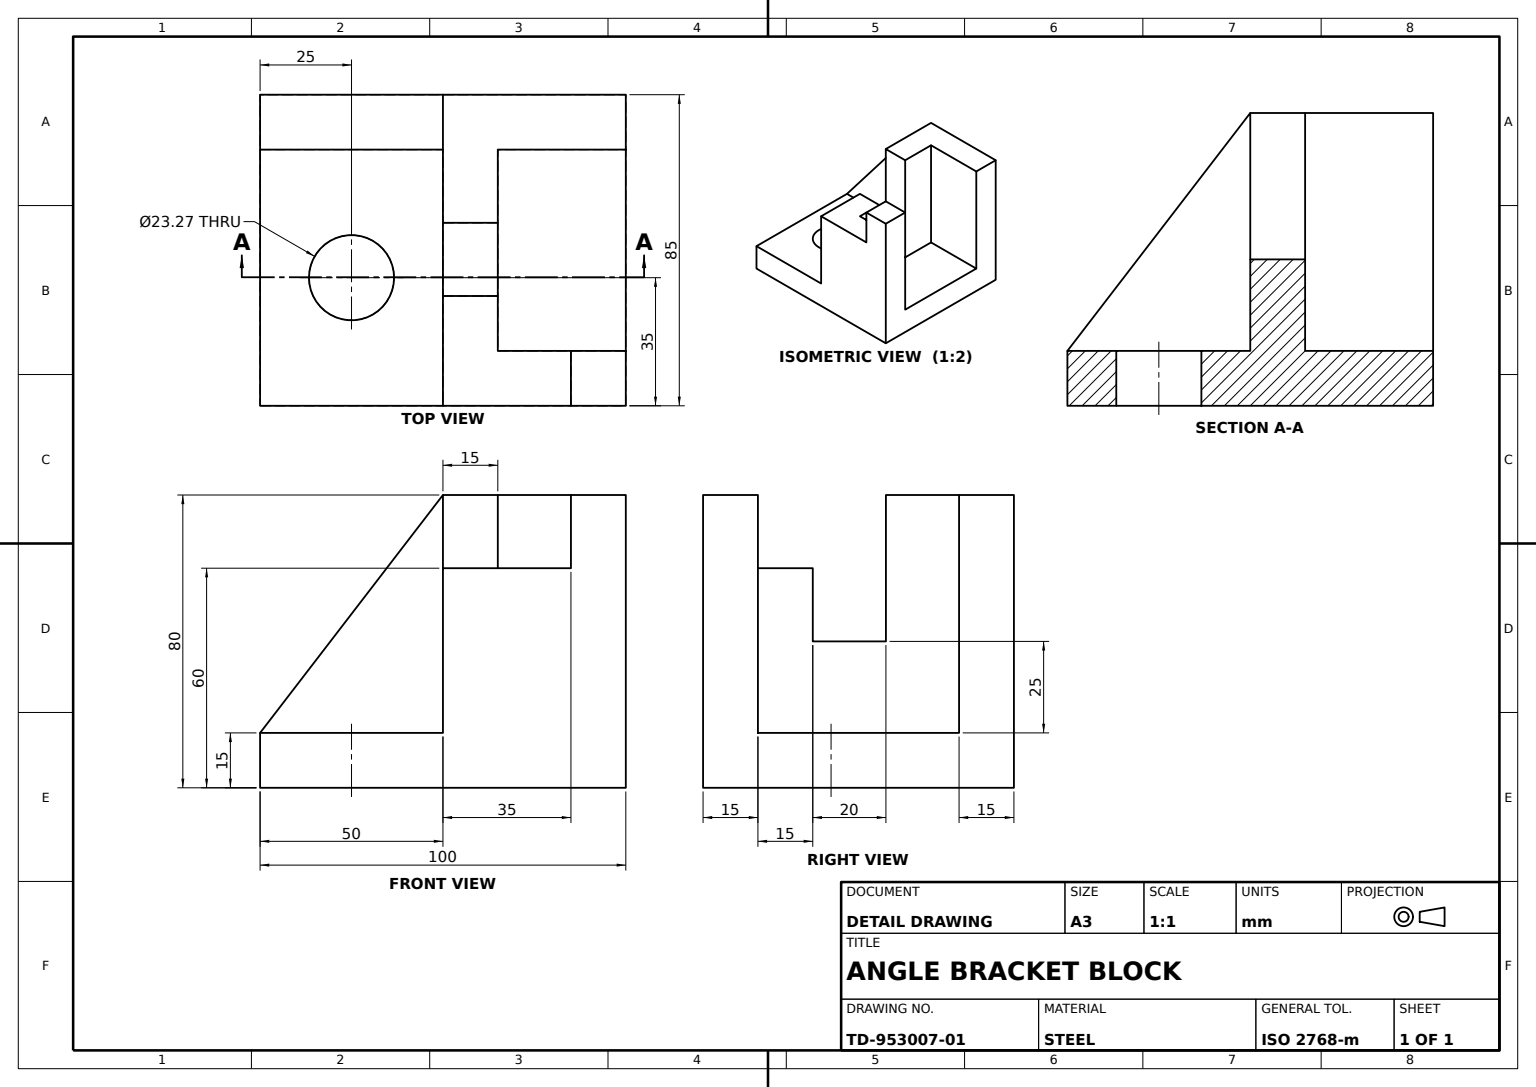
from build123d import *

# Parameters (mm, degrees)
BASE_PLATE_SKETCH_W    = 85
BASE_PLATE_SKETCH_H    = 100
BASE_PLATE_DEPTH       = 15
UPRIGHT_WALL_DEPTH     = 15
SIDE_WALL_SKETCH_W     = 50
SIDE_WALL_SKETCH_H     = 65
SIDE_WALL_DEPTH        = 15
GUSSET_DEPTH           = 15
POST_SKETCH_W          = 20
POST_SKETCH_H          = 15
POST_DEPTH             = 60
STEPPED_BLOCK_DEPTH    = 15
MOUNTING_HOLE_SKETCH_R = 11.636423048
MOUNTING_HOLE_DEPTH    = 15


with BuildPart() as part:
    # Base Plate Sketch → Base Plate (new body)
    with BuildSketch(Plane(origin=(0, 0, 0), x_dir=(1, 0, 0), z_dir=(0, 1, 0))):
        Rectangle(BASE_PLATE_SKETCH_W, BASE_PLATE_SKETCH_H)
    extrude(amount=BASE_PLATE_DEPTH)

    # Upright Wall Sketch → Upright Wall (add)
    with BuildSketch(Plane(origin=(42.5, 0, 0), x_dir=(0, 0, -1), z_dir=(1, 0, 0))):
        Polygon((0, 15), (50, 15), (50, 80), (35, 80), (35, 60), (0, 60), align=None)
    extrude(amount=-UPRIGHT_WALL_DEPTH)

    # Side Wall Sketch → Side Wall (add)
    with BuildSketch(Plane.ZY.offset(42.5)):
        with Locations((-25, 47.5)):
            Rectangle(SIDE_WALL_SKETCH_W, SIDE_WALL_SKETCH_H)
    extrude(amount=-SIDE_WALL_DEPTH)

    # Gusset Sketch → Gusset (add)
    with BuildSketch(Plane.ZY.offset(42.5)):
        Polygon((0, 80), (50, 15), (0, 15), align=None)
    extrude(amount=-GUSSET_DEPTH)

    # Post Sketch → Post (add)
    with BuildSketch(Plane(origin=(0, 80, 0), x_dir=(1, 0, 0), z_dir=(0, 1, 0))):
        with Locations((-17.5, 7.5)):
            Rectangle(POST_SKETCH_W, POST_SKETCH_H)
    extrude(amount=-POST_DEPTH)

    # Stepped Block Sketch → Stepped Block (add)
    with BuildSketch(Plane.XY):
        Polygon((12.5, 40), (12.5, 60), (27.5, 60), (27.5, 15), (-7.5, 15), (-27.5, 14.790865335), (-27.5, 40), (-7.5, 40), align=None)
    extrude(amount=-STEPPED_BLOCK_DEPTH)

    # Mounting Hole Sketch → Mounting Hole (cut)
    with BuildSketch(Plane(origin=(0, 15, 0), x_dir=(1, 0, 0), z_dir=(0, 1, 0))):
        with Locations(Location((7.5, -25, 0), (0, 0, 270))):
            Circle(MOUNTING_HOLE_SKETCH_R)
    extrude(amount=-MOUNTING_HOLE_DEPTH, mode=Mode.SUBTRACT)


solid = part.part
